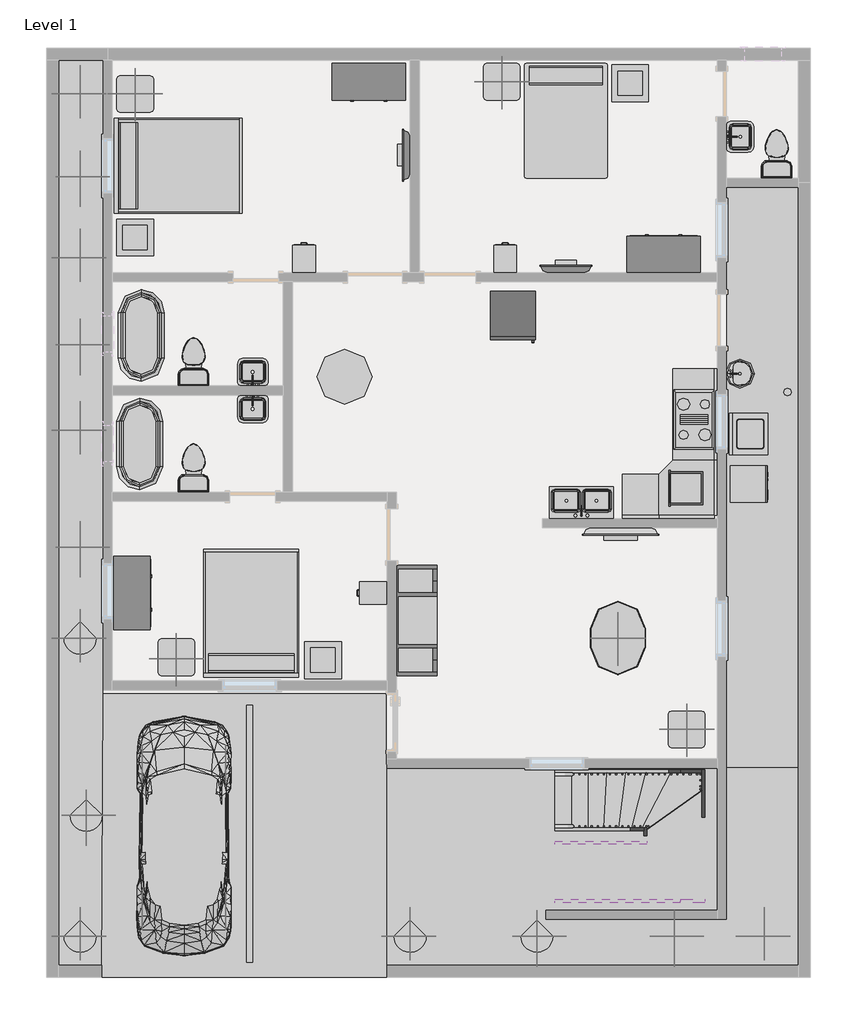
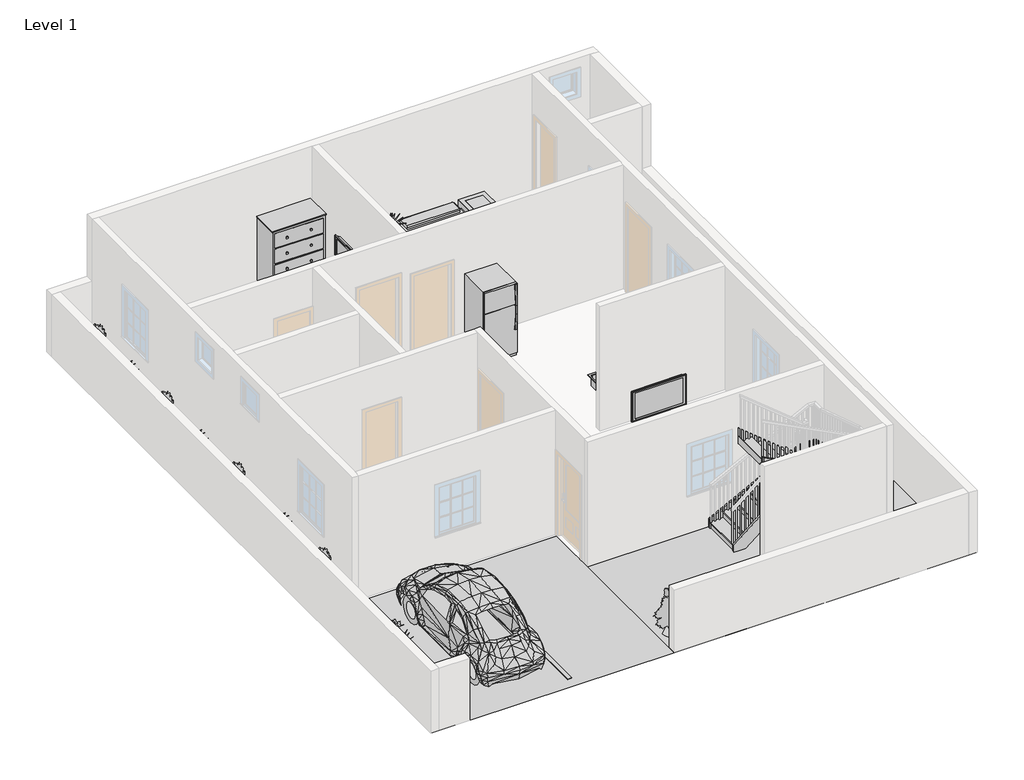
# One storey, part 3 of 3: 23 furniture elements, 18 geographic elements, 14 flow terminals, 11 proxies, 8 members, 1 stair flight.
"""IFC4 building model written with IfcOpenShell, lengths in millimetres."""

from ifc_helpers import new_model, si_unit, frame, origin, place, context, project, spatial, polyline, outline, extrude, triangles, transform, mapped, element, save
from components import proxy_bb1e6e30, proxy_45b28599, proxy_34c9623a, parking_space_9_x_18_90_deg_fdd9e8f5, rpc_beetle_rpc_beetle_3ce7ba48, proxy_a13a33b2, proxy_718fa39f, flow_terminal_accce45a, flow_terminal_a53be723, flow_terminal_d49f872f, flow_terminal_62a433f7, toilet_domestic_3d_toilet_domestic_3d_f7549cf7, toilet_domestic_3d_toilet_domestic_3d_183bbd19, flow_terminal_b374fae2, furniture_35c09872, furniture_0253826f, furniture_bb55ed6b, furniture_9fa109b2, furniture_cf0b6580, furniture_56245f3a, furniture_fdf74506, furniture_b5c51a22, furniture_be1c6672, furniture_905aceb5, furniture_31d08a24, furniture_a415b6c7, rpc_plant_tropical_55f6ff97, rpc_plant_tropical_agave_1_5_93a2a214, rpc_plant_tropical_jungle_flame_3_9c4808c2, stair_flight_927ef07f

model = new_model("IFC4")

# Units and contexts
model_context = context("Model", 3, world=origin())
ifc_project = project(units=[si_unit("LENGTHUNIT", "METRE", prefix="MILLI")], contexts=[model_context])

# Site, building, storey
site = spatial("IfcSite", under=ifc_project)
building = spatial("IfcBuilding", under=site)
storey = spatial("IfcBuildingStorey", under=building, Name="Level 1", Elevation=0.0)

# Proxies
placement = place(None, origin())
element("IfcBuildingElementProxy", 1, Name="Building Element Proxy", at=placement, inside=storey, context=model_context, shape_type="Tessellation", body=[
    triangles([(-12421.2255432, 13336.5010712, 0.0), (-11405.2259308, 13336.5010712, 0.0), (-11506.8255432, -2106.6993164, 0.0), (-12421.2255432, -2106.6993164, 0.0)], [[1, 4, 3], [3, 2, 1]], closed=False),
])
element("IfcBuildingElementProxy", 2, Name="Building Element Proxy", at=placement, inside=storey, context=model_context, shape_type="Tessellation", body=[
    triangles([(-11481.4259308, 2617.7006836, 0.0), (-6776.0753494, 2617.7006836, 0.0), (-6757.0253494, -2106.6993164, 0.0), (-11506.8255432, -2106.6993164, 0.0)], [[1, 4, 3], [3, 2, 1]], closed=False),
])
element("IfcBuildingElementProxy", 3, Name="Building Element Proxy", at=placement, inside=storey, context=model_context, shape_type="Tessellation", body=[
    triangles([(-6757.0253494, 1373.1007805, 0.0), (-6757.0253494, -2106.6993164, 0.0), (278.77459, 1385.4392715, 0.0), (278.77459, -2106.6993164, 0.0)], [[1, 2, 4], [4, 3, 1]], closed=False),
])
element("IfcBuildingElementProxy", 4, Name="Building Element Proxy", at=placement, inside=storey, context=model_context, shape_type="Tessellation", body=[
    triangles([(-1118.2254221, 1373.1007805, 0.0), (278.77459, 1352.1353451, 0.0), (278.77459, 11101.300296, 0.0), (-1118.2254221, 11177.500296, 0.0)], [[4, 1, 3], [2, 3, 1]], closed=False),
])
proxy_shape = proxy_bb1e6e30(model_context)
element("IfcBuildingElementProxy", 5, Name="Cook Top-4 Unit : 36\" x 20\"", ObjectType="Cook Top-4 Unit : 36\" x 20\"", at=placement, inside=storey, context=model_context, shape_type="MappedRepresentation", body=[
    mapped(proxy_shape, transform((-1651.6254019, 7164.3007235, 0.0), x_axis=(0.0, -1.0000000000000004, 0.0), y_axis=(1.0000000000000004, 0.0, 0.0), z_axis=(0.0, 0.0, 1.0))),
])
proxy_2_shape = proxy_45b28599(model_context)
element("IfcBuildingElementProxy", 6, Name="Dishwasher : 24\" x 24\" x 34\"", ObjectType="Dishwasher : 24\" x 24\" x 34\"", at=placement, inside=storey, context=model_context, shape_type="MappedRepresentation", body=[
    mapped(proxy_2_shape, transform((-484.5428704, 5709.517618, 0.0), x_axis=(0.0, 1.000000000000001, 0.0), y_axis=(-1.000000000000001, 0.0, 0.0), z_axis=(0.0, 0.0, 1.0))),
])
proxy_3_shape = proxy_34c9623a(model_context)
element("IfcBuildingElementProxy", 7, Name="Oven Single-Built-in : 21\" x 23 1/2\" x 21\"", ObjectType="Oven Single-Built-in : 21\" x 23 1/2\" x 21\"", at=placement, inside=storey, context=model_context, shape_type="MappedRepresentation", body=[
    mapped(proxy_3_shape, transform((-1919.6912609, 5986.1257962, 762.0), x_axis=(0.0, -1.0000000000000007, 0.0), y_axis=(1.0000000000000007, 0.0, 0.0), z_axis=(0.0, 0.0, 1.0))),
])
parking_space_9_x_18_90_deg_shape = parking_space_9_x_18_90_deg_fdd9e8f5(model_context)
element("IfcBuildingElementProxy", 8, Name="Parking Space : 9' x 18' - 90 deg", ObjectType="Parking Space : 9' x 18' - 90 deg", at=placement, inside=storey, context=model_context, shape_type="MappedRepresentation", body=[
    mapped(parking_space_9_x_18_90_deg_shape, transform((-9043.0254019, -1852.6992765, 0.0), x_axis=(-1.0, 0.0, 0.0), y_axis=(0.0, -1.0, 0.0), z_axis=(0.0, 0.0, 1.0))),
])
rpc_beetle_rpc_beetle_shape = rpc_beetle_rpc_beetle_3ce7ba48(model_context)
element("IfcBuildingElementProxy", 9, Name="RPC Beetle : RPC Beetle", ObjectType="RPC Beetle : RPC Beetle", at=placement, inside=storey, context=model_context, shape_type="MappedRepresentation", body=[
    mapped(rpc_beetle_rpc_beetle_shape, transform((-10135.2254019, -989.0992765, 0.0), x_axis=(1.0, 0.0, 0.0), y_axis=(0.0, 1.0, 0.0), z_axis=(0.0, 0.0, 1.0))),
])
proxy_4_shape = proxy_a13a33b2(model_context)
element("IfcBuildingElementProxy", 10, Name="Refrigerator : 30\" x 32\" RH", ObjectType="Refrigerator : 30\" x 32\" RH", at=placement, inside=storey, context=model_context, shape_type="MappedRepresentation", body=[
    mapped(proxy_4_shape, transform((-4666.2879019, 8909.351752, 0.0), x_axis=(1.0, 0.0, 0.0), y_axis=(0.0, 1.0, 0.0), z_axis=(0.0, 0.0, 1.0))),
])
proxy_5_shape = proxy_718fa39f(model_context)
element("IfcBuildingElementProxy", 11, Name="Washer : 27\" x 25\" x 35\"", ObjectType="Washer : 27\" x 25\" x 35\"", at=placement, inside=storey, context=model_context, shape_type="MappedRepresentation", body=[
    mapped(proxy_5_shape, transform((-470.7758371, 6503.4858162, 0.0), x_axis=(0.0, 1.0000000000000002, 0.0), y_axis=(-1.0000000000000002, 0.0, 0.0), z_axis=(0.0, 0.0, 1.0))),
])

# Flow terminals
flow_terminal_shape = flow_terminal_accce45a(model_context)
element("IfcFlowTerminal", 12, ObjectType="Floor Drain - Round : 5\" Strainer - 2\" Drain", at=placement, inside=storey, context=model_context, shape_type="MappedRepresentation", body=[
    mapped(flow_terminal_shape, transform((-76.8254019, 12091.9007235, 0.0), x_axis=(1.0, 0.0, 0.0), y_axis=(0.0, 1.0, 0.0), z_axis=(0.0, 0.0, 1.0))),
])
element("IfcFlowTerminal", 13, ObjectType="Floor Drain - Round : 5\" Strainer - 2\" Drain", at=placement, inside=storey, context=model_context, shape_type="MappedRepresentation", body=[
    mapped(flow_terminal_shape, transform((-10211.4254019, 9170.9007235, 0.0), x_axis=(1.0, 0.0, 0.0), y_axis=(0.0, 1.0, 0.0), z_axis=(0.0, 0.0, 1.0))),
])
element("IfcFlowTerminal", 14, ObjectType="Floor Drain - Round : 5\" Strainer - 2\" Drain", at=placement, inside=storey, context=model_context, shape_type="MappedRepresentation", body=[
    mapped(flow_terminal_shape, transform((-10287.6254019, 7342.1007235, 0.0), x_axis=(1.0, 0.0, 0.0), y_axis=(0.0, 1.0, 0.0), z_axis=(0.0, 0.0, 1.0))),
])
element("IfcFlowTerminal", 15, ObjectType="Floor Drain - Round : 5\" Strainer - 2\" Drain", at=placement, inside=storey, context=model_context, shape_type="MappedRepresentation", body=[
    mapped(flow_terminal_shape, transform((-102.2254019, 7621.5007235, 0.0), x_axis=(1.0, 0.0, 0.0), y_axis=(0.0, 1.0, 0.0), z_axis=(0.0, 0.0, 1.0))),
])
flow_terminal_2_shape = flow_terminal_a53be723(model_context)
element("IfcFlowTerminal", 16, ObjectType="Sink Kitchen-Double : 42\" x 21\"", at=placement, inside=storey, context=model_context, shape_type="MappedRepresentation", body=[
    mapped(flow_terminal_2_shape, transform((-3511.9313719, 5781.4625839, 0.0), x_axis=(-1.0000000000000002, 0.0, 0.0), y_axis=(0.0, -1.0000000000000002, 0.0), z_axis=(0.0, 0.0, 1.0))),
])
flow_terminal_3_shape = flow_terminal_d49f872f(model_context)
element("IfcFlowTerminal", 17, ObjectType="Sink Vanity-Round : 19\" x 19\"", at=placement, inside=storey, context=model_context, shape_type="MappedRepresentation", body=[
    mapped(flow_terminal_3_shape, transform((-806.9592961, 7829.6489829, 0.0), x_axis=(0.0, 1.0000000000000002, 0.0), y_axis=(-1.0000000000000002, 0.0, 0.0), z_axis=(0.0, 0.0, 1.0))),
])
flow_terminal_4_shape = flow_terminal_62a433f7(model_context)
element("IfcFlowTerminal", 18, ObjectType="Sink Vanity-Square : 20\" x 18\"", at=placement, inside=storey, context=model_context, shape_type="MappedRepresentation", body=[
    mapped(flow_terminal_4_shape, transform((-938.0800008, 11847.6114829, 0.0), x_axis=(0.0, 1.0, 0.0), y_axis=(-1.0, 0.0, 0.0), z_axis=(0.0, 0.0, 1.0))),
])
element("IfcFlowTerminal", 19, ObjectType="Sink Vanity-Square : 20\" x 18\"", at=placement, inside=storey, context=model_context, shape_type="MappedRepresentation", body=[
    mapped(flow_terminal_4_shape, transform((-8976.5361614, 7903.2461246, 0.0), x_axis=(-1.0000000000000004, 0.0, 0.0), y_axis=(0.0, -1.0000000000000004, 0.0), z_axis=(0.0, 0.0, 1.0))),
])
element("IfcFlowTerminal", 20, ObjectType="Sink Vanity-Square : 20\" x 18\"", at=placement, inside=storey, context=model_context, shape_type="MappedRepresentation", body=[
    mapped(flow_terminal_4_shape, transform((-9007.9146425, 7390.5553224, 0.0), x_axis=(1.0, 0.0, 0.0), y_axis=(0.0, 1.0, 0.0), z_axis=(0.0, 0.0, 1.0))),
])
toilet_domestic_3d_toilet_domestic_3d_shape = toilet_domestic_3d_toilet_domestic_3d_f7549cf7(model_context)
toilet_domestic_3d_toilet_domestic_3d_2_shape = toilet_domestic_3d_toilet_domestic_3d_183bbd19(model_context)
element("IfcFlowTerminal", 21, ObjectType="Toilet-Domestic-3D : Toilet-Domestic-3D", at=placement, inside=storey, context=model_context, shape_type="MappedRepresentation", body=[
    mapped(toilet_domestic_3d_toilet_domestic_3d_shape, transform((-280.0254019, 11672.1967509, 0.0), x_axis=(-1.0000000000000004, 0.0, 0.0), y_axis=(0.0, -1.0000000000000004, 0.0), z_axis=(0.0, 0.0, 1.0))),
    mapped(toilet_domestic_3d_toilet_domestic_3d_2_shape, transform((-280.0254019, 11672.1967509, 0.0), x_axis=(-1.0000000000000004, 0.0, 0.0), y_axis=(0.0, -1.0000000000000004, 0.0), z_axis=(0.0, 0.0, 1.0))),
])
element("IfcFlowTerminal", 22, ObjectType="Toilet-Domestic-3D : Toilet-Domestic-3D", at=placement, inside=storey, context=model_context, shape_type="MappedRepresentation", body=[
    mapped(toilet_domestic_3d_toilet_domestic_3d_shape, transform((-9975.9262051, 8217.7967509, 0.0), x_axis=(-1.0000000000000004, 0.0, 0.0), y_axis=(0.0, -1.0000000000000004, 0.0), z_axis=(0.0, 0.0, 1.0))),
    mapped(toilet_domestic_3d_toilet_domestic_3d_2_shape, transform((-9975.9262051, 8217.7967509, 0.0), x_axis=(-1.0000000000000004, 0.0, 0.0), y_axis=(0.0, -1.0000000000000004, 0.0), z_axis=(0.0, 0.0, 1.0))),
])
element("IfcFlowTerminal", 23, ObjectType="Toilet-Domestic-3D : Toilet-Domestic-3D", at=placement, inside=storey, context=model_context, shape_type="MappedRepresentation", body=[
    mapped(toilet_domestic_3d_toilet_domestic_3d_shape, transform((-9975.9262051, 6453.3993121, 0.0), x_axis=(-1.0000000000000004, 0.0, 0.0), y_axis=(0.0, -1.0000000000000004, 0.0), z_axis=(0.0, 0.0, 1.0))),
    mapped(toilet_domestic_3d_toilet_domestic_3d_2_shape, transform((-9975.9262051, 6453.3993121, 0.0), x_axis=(-1.0000000000000004, 0.0, 0.0), y_axis=(0.0, -1.0000000000000004, 0.0), z_axis=(0.0, 0.0, 1.0))),
])
flow_terminal_5_shape = flow_terminal_b374fae2(model_context)
element("IfcFlowTerminal", 24, ObjectType="Tub-Free Standing-3D : 30\" x 60\"", at=placement, inside=storey, context=model_context, shape_type="MappedRepresentation", body=[
    mapped(flow_terminal_5_shape, transform((-10846.4254019, 8561.3007235, 0.0), x_axis=(1.0, 0.0, 0.0), y_axis=(0.0, 1.0, 0.0), z_axis=(0.0, 0.0, 1.0))),
])
element("IfcFlowTerminal", 25, ObjectType="Tub-Free Standing-3D : 30\" x 60\"", at=placement, inside=storey, context=model_context, shape_type="MappedRepresentation", body=[
    mapped(flow_terminal_5_shape, transform((-10871.8254019, 6757.9007235, 0.0), x_axis=(1.0, 0.0, 0.0), y_axis=(0.0, 1.0, 0.0), z_axis=(0.0, 0.0, 1.0))),
])

# Furniture
furniture_shape = furniture_35c09872(model_context)
element("IfcFurniture", 26, ObjectType="Bed-Shaker : Queen 62\" x 83\"", at=placement, inside=storey, context=model_context, shape_type="MappedRepresentation", body=[
    mapped(furniture_shape, transform((-11278.2254019, 11399.7507235, 0.0), x_axis=(0.0, 1.0000000000000002, 0.0), y_axis=(-1.0000000000000002, 0.0, 0.0), z_axis=(0.0, 0.0, 1.0))),
])
element("IfcFurniture", 27, ObjectType="Bed-Shaker : Queen 62\" x 83\"", at=placement, inside=storey, context=model_context, shape_type="MappedRepresentation", body=[
    mapped(furniture_shape, transform((-9036.6754019, 2897.1007235, 0.0), x_axis=(-1.0000000000000002, 0.0, 0.0), y_axis=(0.0, -1.0000000000000002, 0.0), z_axis=(0.0, 0.0, 1.0))),
])
furniture_2_shape = furniture_0253826f(model_context)
element("IfcFurniture", 28, ObjectType="Bed-Standard.0001 : Double 54\" x 75\"", at=placement, inside=storey, context=model_context, shape_type="MappedRepresentation", body=[
    mapped(furniture_2_shape, transform((-4056.7139265, 12175.5958055, 0.0), x_axis=(1.0, 0.0, 0.0), y_axis=(0.0, 1.0, 0.0), z_axis=(0.0, 0.0, 1.0))),
])
furniture_3_shape = furniture_bb55ed6b(model_context)
element("IfcFurniture", 29, ObjectType="Cabinet-File 2 Drawer : 15\" x 18\"", at=placement, inside=storey, context=model_context, shape_type="MappedRepresentation", body=[
    mapped(furniture_3_shape, transform((-8269.221849, 9689.1664234, 0.0), x_axis=(-1.0000000000000002, 0.0, 0.0), y_axis=(0.0, -1.0000000000000002, 0.0), z_axis=(0.0, 0.0, 1.0))),
])
element("IfcFurniture", 30, ObjectType="Cabinet-File 2 Drawer : 15\" x 18\"", at=placement, inside=storey, context=model_context, shape_type="MappedRepresentation", body=[
    mapped(furniture_3_shape, transform((-4922.771849, 9689.1664234, 0.0), x_axis=(-1.0000000000000002, 0.0, 0.0), y_axis=(0.0, -1.0000000000000002, 0.0), z_axis=(0.0, 0.0, 1.0))),
])
element("IfcFurniture", 31, ObjectType="Cabinet-File 2 Drawer : 15\" x 18\"", at=placement, inside=storey, context=model_context, shape_type="MappedRepresentation", body=[
    mapped(furniture_3_shape, transform((-6843.4911018, 4154.4068377, 0.0), x_axis=(0.0, -1.0000000000000002, 0.0), y_axis=(1.0000000000000002, 0.0, 0.0), z_axis=(0.0, 0.0, 1.0))),
])
furniture_4_shape = furniture_9fa109b2(model_context)
element("IfcFurniture", 32, ObjectType="Dresser : 48\" x 72\" x 24\"", at=placement, inside=storey, context=model_context, shape_type="MappedRepresentation", body=[
    mapped(furniture_4_shape, transform((-6792.6321421, 13140.8636776, 0.0), x_axis=(1.0, 0.0, 0.0), y_axis=(0.0, 1.0, 0.0), z_axis=(0.0, 0.0, 1.0))),
])
element("IfcFurniture", 33, ObjectType="Dresser : 48\" x 72\" x 24\"", at=placement, inside=storey, context=model_context, shape_type="MappedRepresentation", body=[
    mapped(furniture_4_shape, transform((-2428.8186618, 9544.3377694, 0.0), x_axis=(-1.0, 0.0, 0.0), y_axis=(0.0, -1.0, 0.0), z_axis=(0.0, 0.0, 1.0))),
])
element("IfcFurniture", 34, ObjectType="Dresser : 48\" x 72\" x 24\"", at=placement, inside=storey, context=model_context, shape_type="MappedRepresentation", body=[
    mapped(furniture_4_shape, transform((-11361.988356, 4551.4965445, 0.0), x_axis=(0.0, 1.0, 0.0), y_axis=(-1.0, 0.0, 0.0), z_axis=(0.0, 0.0, 1.0))),
])
furniture_5_shape = furniture_cf0b6580(model_context)
element("IfcFurniture", 35, ObjectType="Entertainment Center : 72\" x 72\" x 24\"", at=placement, inside=storey, context=model_context, shape_type="MappedRepresentation", body=[
    mapped(furniture_5_shape, transform((-6706.2254019, 3825.1032847, 0.0), x_axis=(0.0, 1.0000000000000002, 0.0), y_axis=(-1.0000000000000002, 0.0, 0.0), z_axis=(0.0, 0.0, 1.0))),
])
furniture_6_shape = furniture_56245f3a(model_context)
element("IfcFurniture", 36, ObjectType="TV - Flat Screen : 32\"", at=placement, inside=storey, context=model_context, shape_type="MappedRepresentation", body=[
    mapped(furniture_6_shape, transform((-6434.5640256, 11554.5562094, 1041.4), x_axis=(0.0, -1.0000000000000004, 0.0), y_axis=(1.0000000000000004, 0.0, 0.0), z_axis=(0.0, 0.0, 1.0))),
])
element("IfcFurniture", 37, ObjectType="TV - Flat Screen : 32\"", at=placement, inside=storey, context=model_context, shape_type="MappedRepresentation", body=[
    mapped(furniture_6_shape, transform((-3789.1699161, 9661.2393472, 914.4), x_axis=(-1.0000000000000004, 0.0, 0.0), y_axis=(0.0, -1.0000000000000004, 0.0), z_axis=(0.0, 0.0, 1.0))),
])
furniture_7_shape = furniture_fdf74506(model_context)
element("IfcFurniture", 38, ObjectType="TV - Flat Screen : 50\"", at=placement, inside=storey, context=model_context, shape_type="MappedRepresentation", body=[
    mapped(furniture_7_shape, transform((-2871.428493, 5307.8285591, 0.0), x_axis=(1.0, 0.0, 0.0), y_axis=(0.0, 1.0, 0.0), z_axis=(0.0, 0.0, 1.0))),
])
furniture_8_shape = furniture_b5c51a22(model_context)
element("IfcFurniture", 39, ObjectType="Table-Coffee : 24\" x 24\" x 24\"", at=placement, inside=storey, context=model_context, shape_type="MappedRepresentation", body=[
    mapped(furniture_8_shape, transform((-10966.2911686, 10091.6896457, 0.0), x_axis=(1.0, 0.0, 0.0), y_axis=(0.0, 1.0, 0.0), z_axis=(0.0, 0.0, 1.0))),
])
element("IfcFurniture", 40, ObjectType="Table-Coffee : 24\" x 24\" x 24\"", at=placement, inside=storey, context=model_context, shape_type="MappedRepresentation", body=[
    mapped(furniture_8_shape, transform((-2736.6911686, 12657.0896457, 0.0), x_axis=(1.0, 0.0, 0.0), y_axis=(0.0, 1.0, 0.0), z_axis=(0.0, 0.0, 1.0))),
])
element("IfcFurniture", 41, ObjectType="Table-Coffee : 24\" x 24\" x 24\"", at=placement, inside=storey, context=model_context, shape_type="MappedRepresentation", body=[
    mapped(furniture_8_shape, transform((-7842.0911686, 3069.4922069, 0.0), x_axis=(1.0, 0.0, 0.0), y_axis=(0.0, 1.0, 0.0), z_axis=(0.0, 0.0, 1.0))),
])
furniture_9_shape = furniture_be1c6672(model_context)
element("IfcFurniture", 42, ObjectType="Table-Dining Oval : 36\" x 48\"", at=placement, inside=storey, context=model_context, shape_type="MappedRepresentation", body=[
    mapped(furniture_9_shape, transform((-3279.7237626, 3933.9203956, 0.0), x_axis=(0.0, 1.0000000000000002, 0.0), y_axis=(-1.0000000000000002, 0.0, 0.0), z_axis=(0.0, 0.0, 1.0))),
])
furniture_10_shape = furniture_905aceb5(model_context)
element("IfcFurniture", 43, ObjectType="Table-Dining Round w Chairs : 36\" Diameter", at=placement, inside=storey, context=model_context, shape_type="MappedRepresentation", body=[
    mapped(furniture_10_shape, transform((-7571.9073691, 8060.379412, 0.0), x_axis=(1.0, 0.0, 0.0), y_axis=(0.0, 1.0, 0.0), z_axis=(0.0, 0.0, 1.0))),
])
furniture_11_shape = furniture_31d08a24(model_context)
element("IfcFurniture", 44, ObjectType="Table-End : 24\" x 24\"", at=placement, inside=storey, context=model_context, shape_type="MappedRepresentation", body=[
    mapped(furniture_11_shape, transform((-11256.5590322, 12422.1007235, 0.0), x_axis=(1.0, 0.0, 0.0), y_axis=(0.0, 1.0, 0.0), z_axis=(0.0, 0.0, 1.0))),
])
element("IfcFurniture", 45, ObjectType="Table-End : 24\" x 24\"", at=placement, inside=storey, context=model_context, shape_type="MappedRepresentation", body=[
    mapped(furniture_11_shape, transform((-5160.5590322, 12625.3007235, 0.0), x_axis=(1.0, 0.0, 0.0), y_axis=(0.0, 1.0, 0.0), z_axis=(0.0, 0.0, 1.0))),
])
element("IfcFurniture", 46, ObjectType="Table-End : 24\" x 24\"", at=placement, inside=storey, context=model_context, shape_type="MappedRepresentation", body=[
    mapped(furniture_11_shape, transform((-10570.7590322, 3063.1032847, 0.0), x_axis=(1.0, 0.0, 0.0), y_axis=(0.0, 1.0, 0.0), z_axis=(0.0, 0.0, 1.0))),
])
element("IfcFurniture", 47, ObjectType="Table-End : 24\" x 24\"", at=placement, inside=storey, context=model_context, shape_type="MappedRepresentation", body=[
    mapped(furniture_11_shape, transform((-2087.1590322, 1862.0507235, 0.0), x_axis=(1.0, 0.0, 0.0), y_axis=(0.0, 1.0, 0.0), z_axis=(0.0, 0.0, 1.0))),
])
furniture_12_shape = furniture_a415b6c7(model_context)
element("IfcFurniture", 48, ObjectType="Work Station Cubicle : 96\" x 96\"", at=placement, inside=storey, context=model_context, shape_type="MappedRepresentation", body=[
    mapped(furniture_12_shape, transform((-1402.3571541, 5023.7441751, 0.0), x_axis=(-0.9999999999999998, 0.0, 0.0), y_axis=(0.0, -0.9999999999999998, 0.0), z_axis=(0.0, 0.0, 1.0))),
])

# Geographic elements
rpc_plant_tropical_shape = rpc_plant_tropical_55f6ff97(model_context)
element("IfcGeographicElement", 49, ObjectType="RPC Plant - Tropical", at=placement, inside=storey, context=model_context, shape_type="MappedRepresentation", body=[
    mapped(rpc_plant_tropical_shape, transform((-11862.4254019, 11202.9007235, 0.0), x_axis=(1.0, 0.0, 0.0), y_axis=(0.0, 1.0, 0.0), z_axis=(0.0, 0.0, 1.0))),
])
element("IfcGeographicElement", 50, ObjectType="RPC Plant - Tropical", at=placement, inside=storey, context=model_context, shape_type="MappedRepresentation", body=[
    mapped(rpc_plant_tropical_shape, transform((-11862.4254019, 8408.9007235, 0.0), x_axis=(1.0, 0.0, 0.0), y_axis=(0.0, 1.0, 0.0), z_axis=(0.0, 0.0, 1.0))),
])
element("IfcGeographicElement", 51, ObjectType="RPC Plant - Tropical", at=placement, inside=storey, context=model_context, shape_type="MappedRepresentation", body=[
    mapped(rpc_plant_tropical_shape, transform((-11862.4254019, 5044.3032847, 0.0), x_axis=(1.0, 0.0, 0.0), y_axis=(0.0, 1.0, 0.0), z_axis=(0.0, 0.0, 1.0))),
])
element("IfcGeographicElement", 52, ObjectType="RPC Plant - Tropical", at=placement, inside=storey, context=model_context, shape_type="MappedRepresentation", body=[
    mapped(rpc_plant_tropical_shape, transform((-4267.8254019, -1420.8992765, 0.0), x_axis=(1.0, 0.0, 0.0), y_axis=(0.0, 1.0, 0.0), z_axis=(0.0, 0.0, 1.0))),
])
element("IfcGeographicElement", 53, ObjectType="RPC Plant - Tropical", at=placement, inside=storey, context=model_context, shape_type="MappedRepresentation", body=[
    mapped(rpc_plant_tropical_shape, transform((-1981.8254019, -1420.8992765, 0.0), x_axis=(1.0, 0.0, 0.0), y_axis=(0.0, 1.0, 0.0), z_axis=(0.0, 0.0, 1.0))),
])
element("IfcGeographicElement", 54, ObjectType="RPC Plant - Tropical", at=placement, inside=storey, context=model_context, shape_type="MappedRepresentation", body=[
    mapped(rpc_plant_tropical_shape, transform((-11760.8254019, 585.7007235, 0.0), x_axis=(1.0, 0.0, 0.0), y_axis=(0.0, 1.0, 0.0), z_axis=(0.0, 0.0, 1.0))),
])
rpc_plant_tropical_agave_1_5_shape = rpc_plant_tropical_agave_1_5_93a2a214(model_context)
element("IfcGeographicElement", 55, ObjectType="RPC Plant - Tropical : Agave - 1.5'", at=placement, inside=storey, context=model_context, shape_type="MappedRepresentation", body=[
    mapped(rpc_plant_tropical_agave_1_5_shape, transform((-10948.0254019, 12574.5007235, 609.6), x_axis=(1.0, 0.0, 0.0), y_axis=(0.0, 1.0, 0.0), z_axis=(0.0, 0.0, 1.0))),
])
element("IfcGeographicElement", 56, ObjectType="RPC Plant - Tropical : Agave - 1.5'", at=placement, inside=storey, context=model_context, shape_type="MappedRepresentation", body=[
    mapped(rpc_plant_tropical_agave_1_5_shape, transform((-4852.0254019, 12777.7007235, 609.6), x_axis=(1.0, 0.0, 0.0), y_axis=(0.0, 1.0, 0.0), z_axis=(0.0, 0.0, 1.0))),
])
element("IfcGeographicElement", 57, ObjectType="RPC Plant - Tropical : Agave - 1.5'", at=placement, inside=storey, context=model_context, shape_type="MappedRepresentation", body=[
    mapped(rpc_plant_tropical_agave_1_5_shape, transform((-10262.2254019, 3190.1032847, 609.6), x_axis=(1.0, 0.0, 0.0), y_axis=(0.0, 1.0, 0.0), z_axis=(0.0, 0.0, 1.0))),
])
element("IfcGeographicElement", 58, ObjectType="RPC Plant - Tropical : Agave - 1.5'", at=placement, inside=storey, context=model_context, shape_type="MappedRepresentation", body=[
    mapped(rpc_plant_tropical_agave_1_5_shape, transform((-1778.6254019, 2014.4507235, 609.6), x_axis=(1.0, 0.0, 0.0), y_axis=(0.0, 1.0, 0.0), z_axis=(0.0, 0.0, 1.0))),
])
element("IfcGeographicElement", 59, ObjectType="RPC Plant - Tropical : Agave - 1.5'", at=placement, inside=storey, context=model_context, shape_type="MappedRepresentation", body=[
    mapped(rpc_plant_tropical_agave_1_5_shape, transform((-2921.6254019, 3532.1007235, 685.8), x_axis=(1.0, 0.0, 0.0), y_axis=(0.0, 1.0, 0.0), z_axis=(0.0, 0.0, 1.0))),
])
rpc_plant_tropical_jungle_flame_3_shape = rpc_plant_tropical_jungle_flame_3_9c4808c2(model_context)
element("IfcGeographicElement", 60, ObjectType="RPC Plant - Tropical : Jungle Flame - 3'", at=placement, inside=storey, context=model_context, shape_type="MappedRepresentation", body=[
    mapped(rpc_plant_tropical_jungle_flame_3_shape, transform((-11862.4254019, 12574.5007235, 0.0), x_axis=(1.0, 0.0, 0.0), y_axis=(0.0, 1.0, 0.0), z_axis=(0.0, 0.0, 1.0))),
])
element("IfcGeographicElement", 61, ObjectType="RPC Plant - Tropical : Jungle Flame - 3'", at=placement, inside=storey, context=model_context, shape_type="MappedRepresentation", body=[
    mapped(rpc_plant_tropical_jungle_flame_3_shape, transform((-11862.4254019, 9856.7007235, 0.0), x_axis=(1.0, 0.0, 0.0), y_axis=(0.0, 1.0, 0.0), z_axis=(0.0, 0.0, 1.0))),
])
element("IfcGeographicElement", 62, ObjectType="RPC Plant - Tropical : Jungle Flame - 3'", at=placement, inside=storey, context=model_context, shape_type="MappedRepresentation", body=[
    mapped(rpc_plant_tropical_jungle_flame_3_shape, transform((-11862.4254019, 6986.5007235, 0.0), x_axis=(1.0, 0.0, 0.0), y_axis=(0.0, 1.0, 0.0), z_axis=(0.0, 0.0, 1.0))),
])
element("IfcGeographicElement", 63, ObjectType="RPC Plant - Tropical : Jungle Flame - 3'", at=placement, inside=storey, context=model_context, shape_type="MappedRepresentation", body=[
    mapped(rpc_plant_tropical_jungle_flame_3_shape, transform((-11862.4254019, 3532.1007235, 0.0), x_axis=(1.0, 0.0, 0.0), y_axis=(0.0, 1.0, 0.0), z_axis=(0.0, 0.0, 1.0))),
])
element("IfcGeographicElement", 64, ObjectType="RPC Plant - Tropical : Jungle Flame - 3'", at=placement, inside=storey, context=model_context, shape_type="MappedRepresentation", body=[
    mapped(rpc_plant_tropical_jungle_flame_3_shape, transform((-11862.4254019, -1420.8992765, 0.0), x_axis=(1.0, 0.0, 0.0), y_axis=(0.0, 1.0, 0.0), z_axis=(0.0, 0.0, 1.0))),
])
element("IfcGeographicElement", 65, ObjectType="RPC Plant - Tropical : Jungle Flame - 3'", at=placement, inside=storey, context=model_context, shape_type="MappedRepresentation", body=[
    mapped(rpc_plant_tropical_jungle_flame_3_shape, transform((-6376.0254019, -1420.8992765, 0.0), x_axis=(1.0, 0.0, 0.0), y_axis=(0.0, 1.0, 0.0), z_axis=(0.0, 0.0, 1.0))),
])
element("IfcGeographicElement", 66, ObjectType="RPC Plant - Tropical : Jungle Flame - 3'", at=placement, inside=storey, context=model_context, shape_type="MappedRepresentation", body=[
    mapped(rpc_plant_tropical_jungle_flame_3_shape, transform((-483.2254019, -1420.8992765, 0.0), x_axis=(1.0, 0.0, 0.0), y_axis=(0.0, 1.0, 0.0), z_axis=(0.0, 0.0, 1.0))),
])

# Members
element("IfcMember", 67, ObjectType="Stringer - 2\" Width", at=placement, inside=storey, context=model_context, shape_type="SweptSolid", body=[
    extrude(outline(polyline([(229.639954, -3966.7570938), (0.0, -3966.7570938), (0.0, -3746.9947762), (962.500629, -1879.3399021), (1305.3956453, -1879.3399021), (229.639954, -3966.7570938)])), frame((0.0, 1296.9007235, 0.0), z_axis=(0.0, 1.0, 0.0), x_axis=(0.0, 0.0, 1.0)), (0.0, 0.0, 1.0), 50.8),
])
element("IfcMember", 68, ObjectType="Stringer - 2\" Width", at=placement, inside=storey, context=model_context, shape_type="SweptSolid", body=[
    extrude(outline(polyline([(-1879.3399021, 1296.9007235), (-1879.3399021, 1347.7007235), (-1524.6254019, 1347.7007235), (-1524.6254019, 1296.9007235), (-1879.3399021, 1296.9007235)])), frame((0.0, 0.0, 962.500629), z_axis=(0.0, 0.0, 1.0), x_axis=(1.0, 0.0, 0.0)), (0.0, 0.0, 1.0), 342.8950162),
])
element("IfcMember", 69, ObjectType="Stringer - 2\" Width", at=placement, inside=storey, context=model_context, shape_type="SweptSolid", body=[
    extrude(outline(polyline([(1347.7007235, 1289.0952212), (1347.7007235, 1000.5956453), (1178.1782405, 1000.5956453), (-811.2992765, 1638.9682298), (-811.2992765, 1969.9972697), (-774.3191592, 1969.9972697), (1347.7007235, 1289.0952212)])), frame((-1524.6254019, 0.0, 0.0), z_axis=(1.0, 0.0, 0.0), x_axis=(0.0, 1.0, 0.0)), (0.0, 0.0, 1.0), 50.8),
])
element("IfcMember", 70, ObjectType="Stringer - 2\" Width", at=placement, inside=storey, context=model_context, shape_type="SweptSolid", body=[
    extrude(outline(polyline([(-1473.8254019, -811.2992765), (-1473.8254019, -862.0992765), (-1879.3399021, -862.0992765), (-1879.3399021, -811.2992765), (-1473.8254019, -811.2992765)])), frame((0.0, 0.0, 1649.8904473), z_axis=(0.0, 0.0, 1.0), x_axis=(1.0, 0.0, 0.0)), (0.0, 0.0, 1.0), 320.1068224),
])
element("IfcMember", 71, ObjectType="Stringer - 2\" Width", at=placement, inside=storey, context=model_context, shape_type="SweptSolid", body=[
    extrude(outline(polyline([(1649.8904473, -1879.3399021), (1969.9972697, -1879.3399021), (3045.7529609, -3966.7570938), (2725.6461385, -3966.7570938), (1649.8904473, -1879.3399021)])), frame((0.0, -862.0992765, 0.0), z_axis=(0.0, 1.0, 0.0), x_axis=(0.0, 0.0, 1.0)), (0.0, 0.0, 1.0), 50.8),
])
element("IfcMember", 72, ObjectType="Stringer - 2\" Width", at=placement, inside=storey, context=model_context, shape_type="SweptSolid", body=[
    extrude(outline(polyline([(176.1764461, -3966.7570938), (0.0, -3966.7570938), (0.0, -3700.4954492), (987.1410923, -2489.8254019), (1380.418648, -2489.8254019), (176.1764461, -3966.7570938)])), frame((0.0, 331.7007235, 0.0), z_axis=(0.0, 1.0, 0.0), x_axis=(0.0, 0.0, 1.0)), (0.0, 0.0, 1.0), 50.8),
])
element("IfcMember", 73, ObjectType="Stringer - 2\" Width", at=placement, inside=storey, context=model_context, shape_type="SweptSolid", body=[
    extrude(outline(polyline([(382.5007235, 1573.2682978), (382.5007235, 1028.5617647), (348.2585062, 1028.5617647), (153.9007235, 1360.465107), (153.9007235, 1926.1409689), (175.8636061, 1926.1409689), (382.5007235, 1573.2682978)])), frame((-2489.8254019, 0.0, 0.0), z_axis=(1.0, 0.0, 0.0), x_axis=(0.0, 1.0, 0.0)), (0.0, 0.0, 1.0), 50.8),
])
element("IfcMember", 74, ObjectType="Stringer - 2\" Width", at=placement, inside=storey, context=model_context, shape_type="SweptSolid", body=[
    extrude(outline(polyline([(1532.8634131, -2439.0254019), (1926.1409689, -2439.0254019), (3171.8038432, -3966.7570938), (2778.5262875, -3966.7570938), (1532.8634131, -2439.0254019)])), frame((0.0, 103.1007235, 0.0), z_axis=(0.0, 1.0, 0.0), x_axis=(0.0, 0.0, 1.0)), (0.0, 0.0, 1.0), 50.8),
])

# Stair flight
stair_flight_shape = stair_flight_927ef07f(model_context)
element("IfcStairFlight", 75, ObjectType="2\" Tread 1\" Nosing 1/4\" Riser", at=placement, inside=storey, context=model_context, shape_type="MappedRepresentation", body=[
    mapped(stair_flight_shape, transform((0.0, 0.0, 0.0), x_axis=(1.0, 0.0, 0.0), y_axis=(0.0, 1.0, 0.0), z_axis=(0.0, 0.0, 1.0))),
])

save(model, "model.ifc")

# Revit data of these elements
# Type "Cook Top-4 Unit : 36\" x 20\""
#   Assembly Code = "E1090400"
#   Depth = 2' - 0"
#   Width = 3' - 0"
#   Burner Material = Steel, Chrome Plated
#   Cooktop Material = Steel, Polished
#   Default Elevation = 0
# Type "Dishwasher : 24\" x 24\" x 34\""
#   Label = "DW"
#   Assembly Code = "E1090400"
#   Depth = 2' - 0"
#   Height = 2' - 10"
#   Width = 2' - 0"
#   Dishwasher Material = Steel, Paint Finish, Ivory, Glossy
#   Panel Face Material = Plastic, Opaque Black
#   Default Elevation = 0
# Type "Oven Single-Built-in : 21\" x 23 1/2\" x 21\""
#   Label = "OVEN"
#   Assembly Code = "E1090400"
#   Depth = 1' - 9"
#   Height = 1' - 11 1/2"
#   Install Height = 0' - 9 1/2"
#   Width = 1' - 9 1/2"
#   Oven Material = Metal - Stainless Steel, Polished
#   Default Elevation = 0
# Type "Parking Space : 9' x 18' - 90 deg"
#   Angle = 90.00°
#   Parking Length = 18' - 0"
#   Parking Width = 9' - 0"
#   pl = 14' - 0"
#   pw = 7' - 0"
# Type "RPC Beetle : RPC Beetle"
#   built-in parameter 1005195 = "RPC-16-0U6E-L4EG-ENH1-J3KF-SVEL-0TX4-C0"
#   Height = 0
# Type "Refrigerator : 30\" x 32\" RH"
#   Label = "REF."
#   Assembly Code = "E1090400"
#   Depth = 2' - 7 3/4"
#   Handle = 2' - 3"
#   Height = 5' - 10"
#   Rear Clearance = 0' - 2"
#   Top Door Height = 1' - 8"
#   Width = 2' - 5 3/8"
#   Material = Carpet (1)
#   Default Elevation = 0
# Type "Washer : 27\" x 25\" x 35\""
#   Label = "W"
#   Assembly Code = "E1090400"
#   Depth = 2' - 1"
#   Height = 2' - 11"
#   Width = 2' - 3"
#   Washer Material = Steel, Paint Finish, Ivory, Matte
#   Default Elevation = 0
# Type "Floor Drain - Round : 5\" Strainer - 2\" Drain"
#   WFU = 2
#   Strainer Height = 0' - 3 1/4"
#   Strainer Radius = 0' - 2 1/2"
#   Strainer Diameter = 0' - 5"
#   Radius 6 = 0' - 0 5/8"
#   Radius 5 = 0' - 1 1/4"
#   Radius 4 = 0' - 1 7/8"
#   Radius 2 = 0' - 3.04167"
#   Radius 1 = 0' - 2.02083"
#   Radius 3 = 0' - 2 1/32"
#   Pipe Radius = 1"
#   Pipe Diameter = 2"
#   Height 2 = 0' - 0.725"
#   Height 1 = 0' - 1 13/16"
#   Body Radius = 0' - 4 1/16"
#   Body Height = 0' - 3 5/8"
#   Body Diameter = 0' - 8 1/8"
#   Drain Material = none
#   HWFU = 0
#   Default Elevation = 0
#   CWFU = 0
# Type "Sink Kitchen-Double : 42\" x 21\""
#   Assembly Code = "D2010410"
#   Counter Height = 3' - 0"
#   Depth = 1' - 9"
#   Width = 3' - 6"
#   Faucet Material = Steel, Polished
#   Sink Material = Steel, Polished
#   Default Elevation = 0
# Type "Sink Vanity-Round : 19\" x 19\""
#   Assembly Code = "D2010400"
#   Top Of Counter = 2' - 7"
#   Basin Material = Porcelain, Linen
#   Faucet Material = Steel, Polished
#   Default Elevation = 0
# Type "Sink Vanity-Square : 20\" x 18\""
#   Assembly Code = "D2010400"
#   Counter Height = 2' - 7"
#   Depth = 1' - 6"
#   Width = 1' - 8"
#   Basin Material = Porcelain, Linen
#   Faucet Material = Steel, Polished
#   Default Elevation = 0
# Type "Toilet-Domestic-3D : Toilet-Domestic-3D"
#   Assembly Code = "D2010110"
#   Toilet - Bowl/Basin Material = Porcelain, Linen
#   Toilet - Seat Material = Laminate, Linen, Matte
#   Default Elevation = 0
# Type "Tub-Free Standing-3D : 30\" x 60\""
#   Assembly Code = "D2010110"
#   Height = 1' - 6"
#   Length = 5' - 0"
#   Width = 2' - 6"
#   Tub Material = Porcelain, Ivory
#   Default Elevation = 0
# Type "Bed-Shaker : Queen 62\" x 83\""
#   Assembly Code = "E2020200"
#   Length = 6' - 11"
#   Width = 5' - 2"
#   Frame Material = Birch
#   Mattress Material = Sash
#   Default Elevation = 0
# Type "Bed-Standard.0001 : Double 54\" x 75\""
#   Assembly Code = "E2020200"
#   Length = 6' - 3"
#   Width = 4' - 6"
#   Leg Material = Steel, Chrome Plated
#   Mattress Material = Linen, White
#   Default Elevation = 0
# Type "Cabinet-File 2 Drawer : 15\" x 18\""
#   Assembly Code = "E2020200"
#   Depth = 1' - 6"
#   Height = 2' - 5"
#   Width = 1' - 3"
#   Cabinet Material = Steel, Paint Finish, Ivory, Glossy
#   Handle Material = Steel, Chrome Plated
#   Default Elevation = 0
# Type "Dresser : 48\" x 72\" x 24\""
#   Assembly Code = "E2020200"
#   Depth = 2' - 0"
#   Height = 6' - 0"
#   Width = 4' - 0"
#   Dresser Material = Wood - Teak
#   Drawer Material = Wood - Teak
#   Knob Material = Cherry
#   Default Elevation = 0
# Type "Entertainment Center : 72\" x 72\" x 24\""
#   Assembly Code = "E2020200"
#   Center Width = 2' - 8"
#   Depth = 2' - 0"
#   Height = 6' - 0"
#   Width = 6' - 0"
#   Material = Wood
#   Default Elevation = 0
# Type "TV - Flat Screen : 32\""
#   SinAng = 0' - 0.0193"
#   L = 2' - 3.79372"
#   H = 1' - 3.6354"
#   Thickness = 0' - 4.33071"
#   Diagonal = 2' - 7.88976"
#   CosAng = 0' - 0.03431"
#   Stand [instance default] = yes
#   Default Elevation = 0
# Type "TV - Flat Screen : 50\""
#   SinAng = 0' - 0.0193"
#   L = 3' - 7.57782"
#   H = 2' - 0.51477"
#   Thickness = 0' - 4.33071"
#   Diagonal = 4' - 2"
#   CosAng = 0' - 0.03431"
#   Stand [instance default] = yes
#   Default Elevation = 0
# Type "Table-Coffee : 24\" x 24\" x 24\""
#   Assembly Code = "E2020200"
#   Height = 2' - 0"
#   Length = 2' - 0"
#   Width = 2' - 0"
#   Top Material = none
#   Frame Material = none
#   Default Elevation = 0
# Type "Table-Dining Oval : 36\" x 48\""
#   Assembly Code = "E2020200"
#   Length = 4' - 0"
#   Width = 3' - 0"
#   Base Material = Steel, Chrome Plated
#   Top Material = Glass - Clear, Grey
#   Default Elevation = 0
#   Description = (empty or 0)
# Type "Table-Dining Round w Chairs : 36\" Diameter"
#   Assembly Code = "E2020200"
#   Radius = 1' - 6"
#   Diameter = 3' - 0"
#   Height = 2' - 6"
#   Chairs = 4
#   Base Material = Pine
#   Top Material = Laminate, Linen, Matte
#   Default Elevation = 0
# Type "Table-End : 24\" x 24\""
#   Assembly Code = "E2020200"
#   Height = 2' - 0"
#   Length = 2' - 0"
#   Width = 2' - 0"
#   Base Material = Birch
#   Top Material = Laminate, Ivory, Matte
#   Default Elevation = 0
# Type "Work Station Cubicle : 96\" x 96\""
#   Assembly Code = "E2020"
#   Desktop Height = 2' - 6"
#   Desktop1 Width = 2' - 3"
#   Desktop2 Width = 2' - 3"
#   Panel Height = 2' - 8"
#   Panel1 Length = 5' - 0"
#   Panel2 Length = 2' - 0"
#   Cube Panel Material = Textile - Light Gray
#   Work Top Material = Laminate, Ivory, Matte
#   Default Elevation = 0
# Type "RPC Plant - Tropical"
#   built-in parameter 1005198 = "{2, 15},{39, RPC-16-FWM5-GM7X-C67P-4000-ST1L-LVER-AU},{1, 0},{1, 0},{2, 13},{1, 8},{5, Color},{1, 0},{1, 0},{3, 0.8},{3, 0.8},{3, 0.8},{1, 8},{7, BBoxMin},{1, 0},{1, 0},{1, 0},{1, 0},{1, 0},{1, 8},{7, BBoxMax},{1, 0},{1, 0},{1, 0},{1, 0},{1, 0},{2, 11},{9, RPCTypeId},{1, 0},{1, 0},{39, RPC-16-FWM5-GM7X-C67P-4000-ST1L-LVER-AU},{1, 6},{14, RPCPlantHeight},{1, 0},{1, 0},{1, 3},{2, 11},{7, keyword},{1, 0},{1, 0},{35, :RPCs:Shrubs [General]:Geometry:RPC},{2, 11},{8, category},{1, 0},{1, 0},{16, Shrubs [General]},{2, 11},{12, LocalizedUID},{1, 0},{1, 0},{10, Crane Lily},{2, 14},{6, Height},{1, 0},{1, 0},{1, 3},{1, 2},{16, Cast Reflections},{1, 0},{1, 0},{1, 0},{1, 2},{12, Cast Shadows},{1, 0},{1, 0},{1, 1},{1, 2},{9, Lock View},{1, 0},{1, 0},{1, 0},{1, 4},{5, ViewC},{1, 0},{1, 0},{1, 0},{21, assetlibrary_base.fbx},{1, 5},"
#   built-in parameter 1005195 = "RPC-16-FWM5-GM7X-C67P-4000-ST1L-LVER-AU"
#   Assembly Code = "G2050500"
#   Height = 3' - 0"
#   Default Elevation = 0
# Type "RPC Plant - Tropical : Agave - 1.5'"
#   built-in parameter 1005198 = "{2, 15},{39, RPC-16-G1GJ-63FX-7K5P-N000-ST1L-LVER-AU},{1, 0},{1, 0},{2, 13},{1, 8},{5, Color},{1, 0},{1, 0},{3, 0.8},{3, 0.8},{3, 0.8},{1, 8},{7, BBoxMin},{1, 0},{1, 0},{1, 0},{1, 0},{1, 0},{1, 8},{7, BBoxMax},{1, 0},{1, 0},{1, 0},{1, 0},{1, 0},{2, 11},{9, RPCTypeId},{1, 0},{1, 0},{39, RPC-16-G1GJ-63FX-7K5P-N000-ST1L-LVER-AU},{1, 6},{14, RPCPlantHeight},{1, 0},{1, 0},{3, 1.5},{2, 11},{7, keyword},{1, 0},{1, 0},{35, :RPCs:Plants [General]:Geometry:RPC},{2, 11},{8, category},{1, 0},{1, 0},{16, Plants [General]},{2, 11},{12, LocalizedUID},{1, 0},{1, 0},{5, Agave},{2, 14},{6, Height},{1, 0},{1, 0},{3, 1.5},{1, 2},{16, Cast Reflections},{1, 0},{1, 0},{1, 0},{1, 2},{12, Cast Shadows},{1, 0},{1, 0},{1, 1},{1, 2},{9, Lock View},{1, 0},{1, 0},{1, 0},{1, 4},{5, ViewC},{1, 0},{1, 0},{1, 0},{21, assetlibrary_base.fbx},{1, 5},"
#   built-in parameter 1005195 = "RPC-16-G1GJ-63FX-7K5P-N000-ST1L-LVER-AU"
#   Type Comments = "Agave"
#   Assembly Code = "G2050500"
#   Height = 1' - 6"
#   Default Elevation = 0
# Type "RPC Plant - Tropical : Jungle Flame - 3'"
#   built-in parameter 1005198 = "{2, 15},{39, RPC-16-FUVJ-JWG0-MWGK-8000-ST1L-LVER-AU},{1, 0},{1, 0},{2, 13},{1, 8},{5, Color},{1, 0},{1, 0},{3, 0.8},{3, 0.8},{3, 0.8},{1, 8},{7, BBoxMin},{1, 0},{1, 0},{1, 0},{1, 0},{1, 0},{1, 8},{7, BBoxMax},{1, 0},{1, 0},{1, 0},{1, 0},{1, 0},{2, 11},{9, RPCTypeId},{1, 0},{1, 0},{39, RPC-16-FUVJ-JWG0-MWGK-8000-ST1L-LVER-AU},{1, 6},{14, RPCPlantHeight},{1, 0},{1, 0},{1, 3},{2, 11},{7, keyword},{1, 0},{1, 0},{35, :RPCs:Shrubs [General]:Geometry:RPC},{2, 11},{8, category},{1, 0},{1, 0},{16, Shrubs [General]},{2, 11},{12, LocalizedUID},{1, 0},{1, 0},{12, Jungle Flame},{2, 14},{6, Height},{1, 0},{1, 0},{1, 3},{1, 2},{16, Cast Reflections},{1, 0},{1, 0},{1, 0},{1, 2},{12, Cast Shadows},{1, 0},{1, 0},{1, 1},{1, 2},{9, Lock View},{1, 0},{1, 0},{1, 0},{1, 4},{5, ViewC},{1, 0},{1, 0},{1, 0},{21, assetlibrary_base.fbx},{1, 5},"
#   built-in parameter 1005195 = "RPC-16-FUVJ-JWG0-MWGK-8000-ST1L-LVER-AU"
#   Type Comments = "Jungle Flame"
#   Assembly Code = "G2050500"
#   Height = 3' - 0"
#   Default Elevation = 0
# Elements 1, 2, 3, 4 (IfcBuildingElementProxy)
#   Material = Plant
#   Phase Created = New Construction
# Element 5 (IfcBuildingElementProxy, "Cook Top-4 Unit : 36\" x 20\"")
#   Phase Created = New Construction
#   Materials on its faces: "Steel, Chrome Plated", "Steel, Polished"
# Element 6 (IfcBuildingElementProxy, "Dishwasher : 24\" x 24\" x 34\"")
#   Phase Created = New Construction
#   Materials on its faces: "Steel, Paint Finish, Ivory, Glossy", "Plastic, Opaque Black"
# Element 7 (IfcBuildingElementProxy, "Oven Single-Built-in : 21\" x 23 1/2\" x 21\"")
#   Phase Created = New Construction
#   Materials on its faces: "Steel", "Metal - Stainless Steel, Polished", "Glass"
# Element 8 (IfcBuildingElementProxy, "Parking Space : 9' x 18' - 90 deg")
#   Phase Created = New Construction
#   Materials on its faces: "Parking Stripe"
# Element 9 (IfcBuildingElementProxy, "RPC Beetle : RPC Beetle")
#   Phase Created = New Construction
# Element 10 (IfcBuildingElementProxy, "Refrigerator : 30\" x 32\" RH")
#   Phase Created = New Construction
#   Materials on its faces: "Carpet (1)", "Steel, Chrome Plated"
# Element 11 (IfcBuildingElementProxy, "Washer : 27\" x 25\" x 35\"")
#   Phase Created = New Construction
#   Materials on its faces: "Steel, Paint Finish, Ivory, Matte"
# Element 12 (IfcFlowTerminal, "Floor Drain - Round : 5\" Strainer - 2\" Drain")
#   Mark = "3"
#   Phase Created = New Construction
# Element 13 (IfcFlowTerminal, "Floor Drain - Round : 5\" Strainer - 2\" Drain")
#   Mark = "6"
#   Phase Created = New Construction
# Element 14 (IfcFlowTerminal, "Floor Drain - Round : 5\" Strainer - 2\" Drain")
#   Mark = "11"
#   Phase Created = New Construction
# Element 15 (IfcFlowTerminal, "Floor Drain - Round : 5\" Strainer - 2\" Drain")
#   Mark = "14"
#   Phase Created = New Construction
# Element 16 (IfcFlowTerminal, "Sink Kitchen-Double : 42\" x 21\"")
#   Mark = "12"
#   Phase Created = New Construction
#   Materials on its faces: "Steel, Polished"
# Element 17 (IfcFlowTerminal, "Sink Vanity-Round : 19\" x 19\"")
#   Mark = "13"
#   Phase Created = New Construction
#   Materials on its faces: "Porcelain, Linen", "Steel, Polished"
# Element 18 (IfcFlowTerminal, "Sink Vanity-Square : 20\" x 18\"")
#   Mark = "2"
#   Phase Created = New Construction
#   Materials on its faces: "Porcelain, Linen", "Steel, Polished"
# Element 19 (IfcFlowTerminal, "Sink Vanity-Square : 20\" x 18\"")
#   Mark = "7"
#   Phase Created = New Construction
#   Materials on its faces: "Porcelain, Linen", "Steel, Polished"
# Element 20 (IfcFlowTerminal, "Sink Vanity-Square : 20\" x 18\"")
#   Mark = "10"
#   Phase Created = New Construction
#   Materials on its faces: "Porcelain, Linen", "Steel, Polished"
# Element 21 (IfcFlowTerminal, "Toilet-Domestic-3D : Toilet-Domestic-3D")
#   Mark = "1"
#   Phase Created = New Construction
#   Materials on its faces: "Porcelain, Linen", "Laminate, Linen, Matte"
# Element 22 (IfcFlowTerminal, "Toilet-Domestic-3D : Toilet-Domestic-3D")
#   Mark = "4"
#   Phase Created = New Construction
#   Materials on its faces: "Porcelain, Linen", "Laminate, Linen, Matte"
# Element 23 (IfcFlowTerminal, "Toilet-Domestic-3D : Toilet-Domestic-3D")
#   Mark = "9"
#   Phase Created = New Construction
#   Materials on its faces: "Porcelain, Linen", "Laminate, Linen, Matte"
# Element 24 (IfcFlowTerminal, "Tub-Free Standing-3D : 30\" x 60\"")
#   Mark = "5"
#   Phase Created = New Construction
#   Materials on its faces: "Porcelain, Ivory"
# Element 25 (IfcFlowTerminal, "Tub-Free Standing-3D : 30\" x 60\"")
#   Mark = "8"
#   Phase Created = New Construction
#   Materials on its faces: "Porcelain, Ivory"
# Elements 26, 27 (IfcFurniture, "Bed-Shaker : Queen 62\" x 83\"")
#   Phase Created = New Construction
#   Materials on its faces: "Birch", "Sash"
# Element 28 (IfcFurniture, "Bed-Standard.0001 : Double 54\" x 75\"")
#   Phase Created = New Construction
#   Materials on its faces: "Linen, White", "Steel, Chrome Plated"
# Elements 29, 30, 31 (IfcFurniture, "Cabinet-File 2 Drawer : 15\" x 18\"")
#   Phase Created = New Construction
#   Materials on its faces: "Steel, Chrome Plated", "Steel, Paint Finish, Ivory, Glossy"
# Elements 32, 33, 34 (IfcFurniture, "Dresser : 48\" x 72\" x 24\"")
#   Phase Created = New Construction
#   Materials on its faces: "Laminate, Ivory, Matte", "Cherry", "Wood - Teak"
# Element 35 (IfcFurniture, "Entertainment Center : 72\" x 72\" x 24\"")
#   Phase Created = New Construction
#   Materials on its faces: "Wood", "Steel, Chrome Plated", "Glass - Clear, Grey"
# Elements 36, 37 (IfcFurniture, "TV - Flat Screen : 32\"")
#   Stand = yes
#   Phase Created = New Construction
#   Materials on its faces: "TV - Black", "TV - Glass", "TV - Screen"
# Element 38 (IfcFurniture, "TV - Flat Screen : 50\"")
#   Stand = yes
#   Phase Created = New Construction
#   Materials on its faces: "TV - Black", "TV - Glass", "TV - Screen"
# Elements 39, 40, 41 (IfcFurniture, "Table-Coffee : 24\" x 24\" x 24\"")
#   Phase Created = New Construction
#   Materials on its faces: "Glass - Clear, Grey"
# Element 42 (IfcFurniture, "Table-Dining Oval : 36\" x 48\"")
#   Phase Created = New Construction
#   Materials on its faces: "Steel, Chrome Plated", "Glass - Clear, Grey"
# Element 43 (IfcFurniture, "Table-Dining Round w Chairs : 36\" Diameter")
#   Phase Created = New Construction
#   Materials on its faces: "Pine", "Laminate, Linen, Matte"
# Elements 44, 45, 46, 47 (IfcFurniture, "Table-End : 24\" x 24\"")
#   Phase Created = New Construction
#   Materials on its faces: "Laminate, Ivory, Matte", "Birch"
# Element 48 (IfcFurniture, "Work Station Cubicle : 96\" x 96\"")
#   Phase Created = New Construction
#   Materials on its faces: "Textile - Light Gray", "Laminate, Ivory, Matte"
# Elements 49, 50, 51, 52, 53, 54 (IfcGeographicElement, "RPC Plant - Tropical")
#   Phase Created = New Construction
# Elements 55, 56, 57, 58, 59 (IfcGeographicElement, "RPC Plant - Tropical : Agave - 1.5'")
#   Phase Created = New Construction
# Elements 60, 61, 62, 63, 64, 65, 66 (IfcGeographicElement, "RPC Plant - Tropical : Jungle Flame - 3'")
#   Phase Created = New Construction
# Elements 67, 68, 69, 70, 71, 72, 73, 74 (IfcMember, "Stringer - 2\" Width")
#   Phase Created = New Construction
# Element 75 (IfcStairFlight, "2\" Tread 1\" Nosing 1/4\" Riser")
#   Phase Created = New Construction
# Materials
#   "Steel, Chrome Plated": class "Metal", colour RGB 17 17 17, transparency 0, Description = "Chromiuim plated steel", Cost = 0
#   "Steel, Polished": class "Metal", colour RGB 57 57 57, transparency 0, Description = "Polished steel", Cost = 0
#   "Steel, Paint Finish, Ivory, Glossy": class "Metal", colour RGB 247 247 239, transparency 0, Description = "Steel, paint finish, ivory, glossy", Cost = 0
#   "Plastic, Opaque Black": class "Plastic", colour RGB 0 0 0, transparency 0.7, Description = "Plastic, generic, opaque black", Cost = 0
#   "Metal - Stainless Steel, Polished": class "Metal", colour RGB 215 215 215, transparency 0
#   "Carpet (1)": class "Carpet", colour RGB 124 80 67, transparency 0, Description = "Interior finish"
#   "Steel, Paint Finish, Ivory, Matte": class "Metal", colour RGB 247 247 239, transparency 0, Description = "Steel, paint finish, ivory, matte", Cost = 0
#   "Porcelain, Linen": class "Ceramic", colour RGB 249 239 230, transparency 0, Description = "Porcelain, linen", Cost = 0
#   "Laminate, Linen, Matte": class "Plastic", colour RGB 249 239 230, transparency 0, Description = "Plastic Laminate - Linen, Matte", Cost = 0
#   "Porcelain, Ivory": class "Ceramic", colour RGB 247 247 239, transparency 0, Description = "Porcelain, ivory", Cost = 0
#   "Birch": class "Wood", colour RGB 224 178 126, transparency 0, Description = "Betula Alleghaniensis", Cost = 0
#   "Sash": class "Wood", colour RGB 224 178 126, transparency 0
#   "Linen, White": class "Textile", colour RGB 247 247 239, transparency 0, Description = "Linen, white", Cost = 0
#   "Wood - Teak": class "Wood", colour RGB 145 112 90, transparency 0
#   "Cherry": class "Wood", colour RGB 226 177 128, transparency 0, Description = "Prunus Serotina", Cost = 0
#   "Wood": class "Wood", colour RGB 0 0 0, transparency 0, Description = "Generic wood", Cost = 0
#   "Glass - Clear, Grey": class "Glass", colour RGB 252 255 255, transparency 0.64
#   "Pine": class "Wood", colour RGB 223 192 134, transparency 0, Description = "Pinus Echinata", Cost = 0
#   "Laminate, Ivory, Matte": class "Plastic", colour RGB 247 247 239, transparency 0, Description = "Plastic Laminate - Ivory, Matte", Cost = 0
#   "Textile - Light Gray": class "Fabric", colour RGB 204 204 204, transparency 0
#   "Plant": class "Generic", colour RGB 0 0 0, transparency 0, Description = "physical material", Cost = 0
#   "Steel": class "Metal", colour RGB 247 247 247, transparency 0, Description = "Steel, mill finish", Cost = 0
#   "Glass": class "Glass", colour RGB 0 128 192, transparency 0.75, Description = "Soda Lime Glass", Cost = 0
#   "Parking Stripe": class "Paint", colour RGB 250 250 91, transparency 0
#   "TV - Black": colour RGB 49 49 49, transparency 0
#   "TV - Glass": colour RGB 157 157 157, transparency 0.9
#   "TV - Screen": colour RGB 0 0 0, transparency 0
